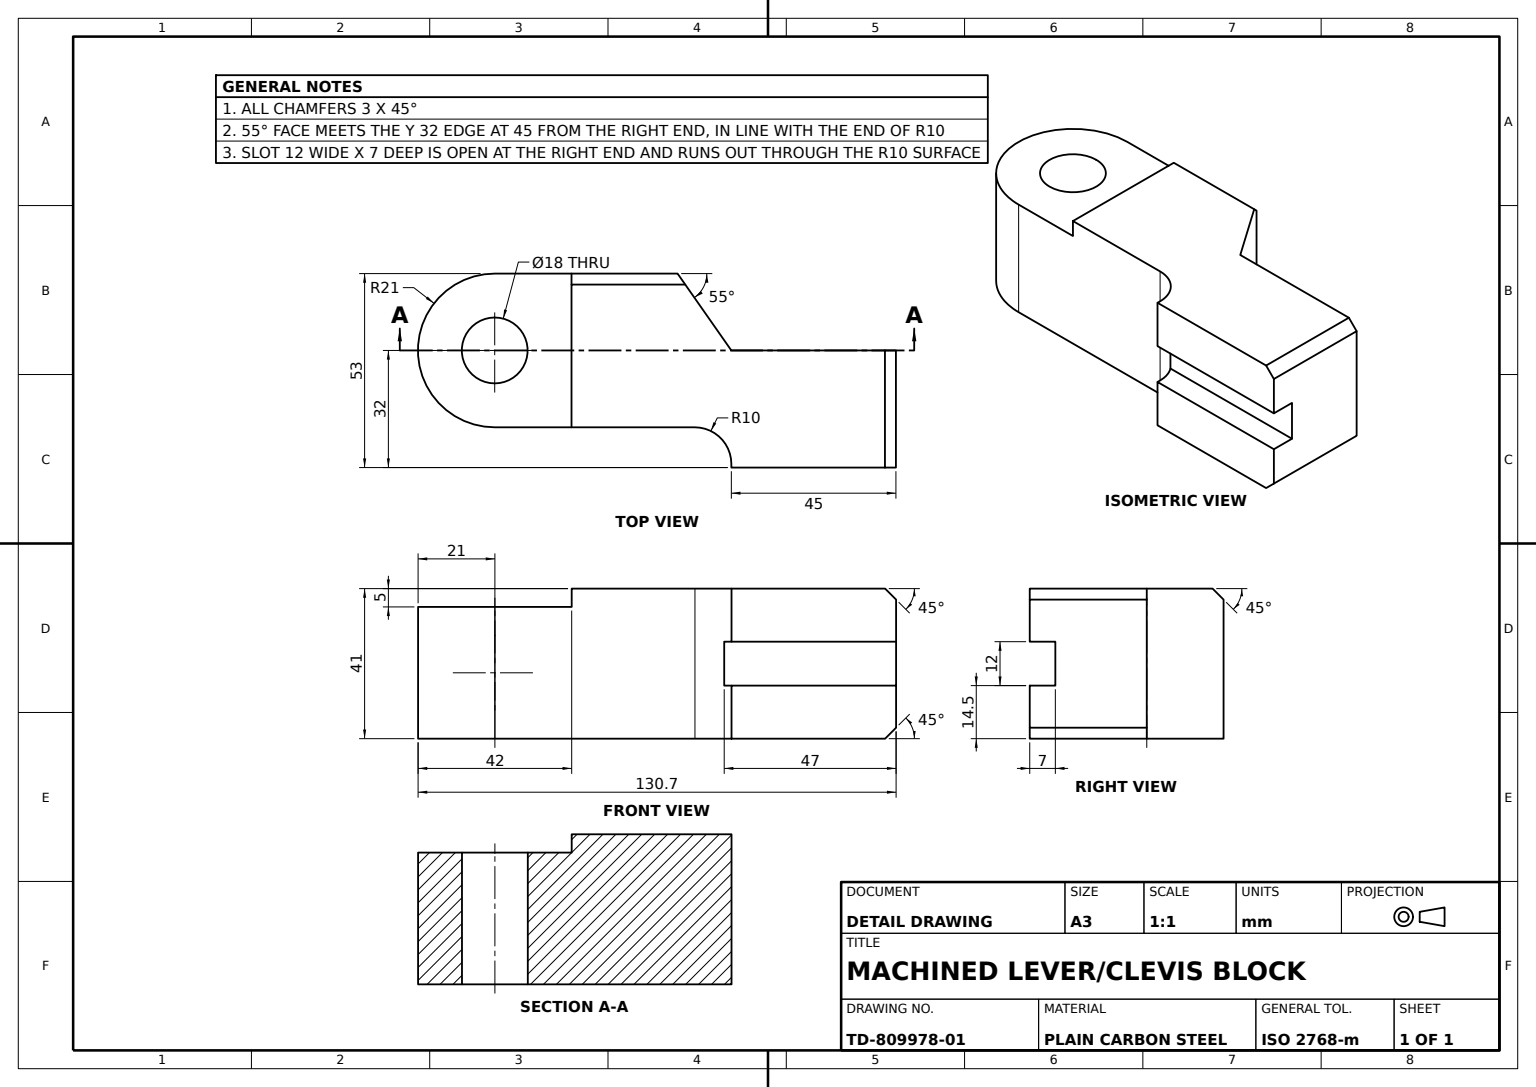
from build123d import *

# Parameters (mm, degrees)
LINK_PROFILE_SKETCH_R    = 9
LINK_BODY_DEPTH          = 20.5
EYE_RECESS_CUT_5MM_DEPTH = 5
SLOT_SKETCH_W            = 14
SLOT_SKETCH_H            = 12
SLOT_CUT_14X12_DEPTH     = 75
END_CHAMFER_3MM_SIZE     = 3


with BuildPart() as part:
    # Link Profile Sketch → Link Body (new, symmetric)
    with BuildSketch(Plane(origin=(0, 0, 0), x_dir=(1, 0, 0), z_dir=(0, 1, 0))):
        with BuildLine():
            Line((9.704358302, -32), (54.704358302, -32))
            Line((54.704358302, -32), (54.704358302, 0))
            Line((54.704358302, 0), (9.704358302, 0))
            Line((9.704358302, 0), (-5, 21))
            Line((-5, 21), (-55, 21))
            ThreePointArc((-55, 21), (-76, 0), (-55, -21))
            Line((-55, -21), (-0.295641698, -21))
            ThreePointArc((-0.295641698, -21), (6.775426114, -23.928932188), (9.704358302, -31))
            Line((9.704358302, -31), (9.704358302, -32))
        make_face()
        with Locations(Location((-55, 0, 0), (0, 0, 270))):
            Circle(LINK_PROFILE_SKETCH_R, mode=Mode.SUBTRACT)
    extrude(amount=LINK_BODY_DEPTH, both=True)

    # Eye Recess Sketch → Eye Recess Cut 5mm (cut)
    with BuildSketch(Plane(origin=(0, 20.5, 0), x_dir=(1, 0, 0), z_dir=(0, 1, 0))):
        with BuildLine():
            Line((-55, -21), (-34, -21))
            Line((-34, -21), (-34, 21))
            Line((-34, 21), (-55, 21))
            ThreePointArc((-55, 21), (-76, 0), (-55, -21))
        make_face()
    extrude(amount=-EYE_RECESS_CUT_5MM_DEPTH, mode=Mode.SUBTRACT)

    # Slot Sketch → Slot Cut 14x12 (cut)
    with BuildSketch(Plane(origin=(54.704358302, 0, 0), x_dir=(0, 0, -1), z_dir=(1, 0, 0))):
        with Locations((-32, 0)):
            Rectangle(SLOT_SKETCH_W, SLOT_SKETCH_H)
    extrude(amount=-SLOT_CUT_14X12_DEPTH, mode=Mode.SUBTRACT)

    # End Chamfer 3mm
    end_chamfer_3mm_edges = [part.edges().sort_by_distance(p)[0] for p in [
        (54.704358302, -20.5, 16),
        (-19.5, 20.5, -21),
        (54.704358302, 20.5, 16),
    ]]
    chamfer(end_chamfer_3mm_edges, length=END_CHAMFER_3MM_SIZE)


solid = part.part
